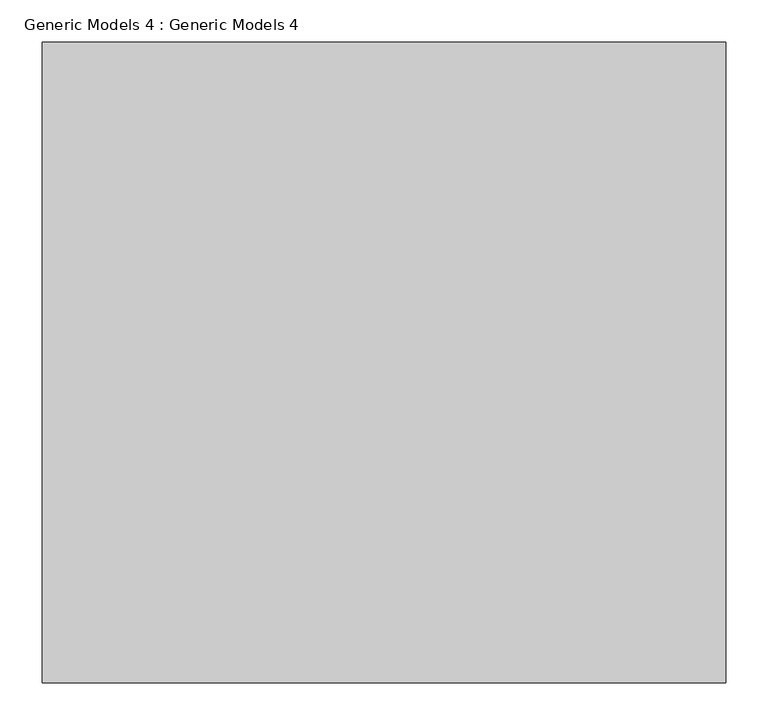
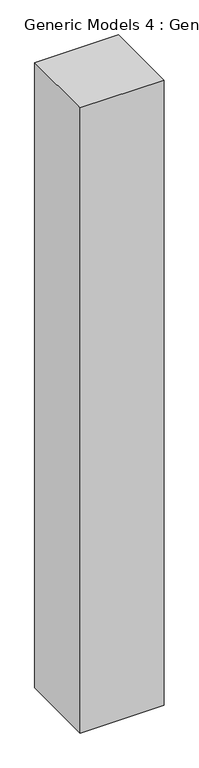
"""IFC4 building model written with IfcOpenShell, lengths in millimetres: proxy geometry, Generic Models 4 : Generic Models 4."""

from ifc_helpers import new_model, si_unit, origin, origin_with_axes, place, context, project, spatial, polyline, outline, extrude, source, transform, mapped, element, save


def generic_models_4_generic_models_4_105e3c89(model_context):
    return source(origin(), model_context, "Body", "SweptSolid", [
        extrude(outline(polyline([(-9650.4069895, -8492.7980299), (-9650.4069895, -9254.7980299), (-10463.2069895, -9254.7980299), (-10463.2069895, -8492.7980299), (-9650.4069895, -8492.7980299)])), origin_with_axes(), (0.0, 0.0, 1.0), 6396.0043662),
    ])


if __name__ == "__main__":
    model = new_model("IFC4")
    model_context = context("Model", 3, world=origin())
    ifc_project = project(units=[si_unit("LENGTHUNIT", "METRE", prefix="MILLI")], contexts=[model_context])
    site = spatial("IfcSite", under=ifc_project)
    building = spatial("IfcBuilding", under=site)
    placement = place(None, origin())
    generic_models_4_generic_models_4_shape = generic_models_4_generic_models_4_105e3c89(model_context)
    element("IfcBuildingElementProxy", 1, Name="Generic Models 4 : Generic Models 4", ObjectType="Generic Models 4 : Generic Models 4", at=placement, inside=building, context=model_context, shape_type="MappedRepresentation", body=[
        mapped(generic_models_4_generic_models_4_shape, transform((0.0, 0.0, 0.0), x_axis=(1.0, 0.0, 0.0), y_axis=(0.0, 1.0, 0.0), z_axis=(0.0, 0.0, 1.0))),
    ])
    save(model, "model.ifc")
